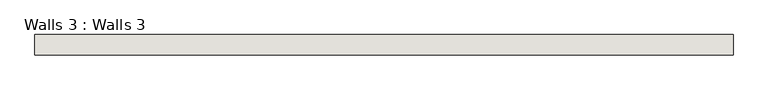
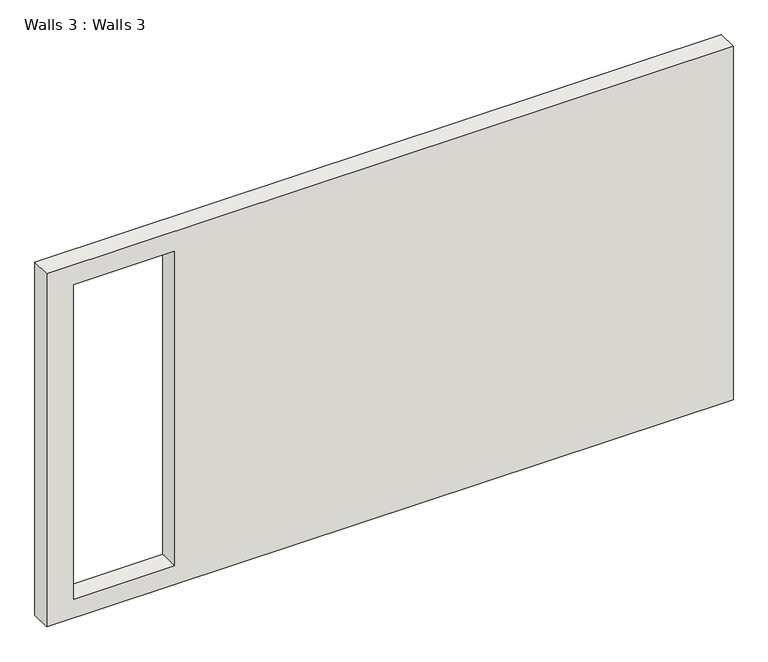
"""IFC4 building model written with IfcOpenShell, lengths in millimetres: wall geometry, Walls 3 : Walls 3."""

from ifc_helpers import new_model, si_unit, frame, origin, place, context, project, spatial, polyline, outline, extrude, source, transform, mapped, element, save


def walls_3_walls_3_a1481ceb(model_context):
    return source(origin(), model_context, "Body", "SweptSolid", [
        extrude(outline(polyline([(5648.0, -7329.4383357), (5648.0, -17716.4633774), (0.0, -17716.4633774), (0.0, -7329.4383357), (5648.0, -7329.4383357)]), holes=[polyline([(5328.8432697, -15781.5417193), (299.6432697, -15781.5417193), (299.6432697, -17305.5417193), (5328.8432697, -17305.5417193), (5328.8432697, -15781.5417193)])]), frame((0.0, -20435.7210337, 0.0), z_axis=(0.0, 1.0, 0.0), x_axis=(0.0, 0.0, 1.0)), (0.0, 0.0, 1.0), 304.8),
    ])


if __name__ == "__main__":
    model = new_model("IFC4")
    model_context = context("Model", 3, world=origin())
    ifc_project = project(units=[si_unit("LENGTHUNIT", "METRE", prefix="MILLI")], contexts=[model_context])
    site = spatial("IfcSite", under=ifc_project)
    building = spatial("IfcBuilding", under=site)
    placement = place(None, origin())
    walls_3_walls_3_shape = walls_3_walls_3_a1481ceb(model_context)
    element("IfcWall", 1, ObjectType="Walls 3 : Walls 3", at=placement, inside=building, context=model_context, shape_type="MappedRepresentation", body=[
        mapped(walls_3_walls_3_shape, transform((0.0, 0.0, 0.0), x_axis=(1.0, 0.0, 0.0), y_axis=(0.0, 1.0, 0.0), z_axis=(0.0, 0.0, 1.0))),
    ])
    save(model, "model.ifc")

# Revit data of these elements
# Element 1 (IfcWall, "Walls 3 : Walls 3")
#   Materials on its faces: "Default Wall"
# Materials
#   "Default Wall": colour RGB 80 80 80, transparency 0
